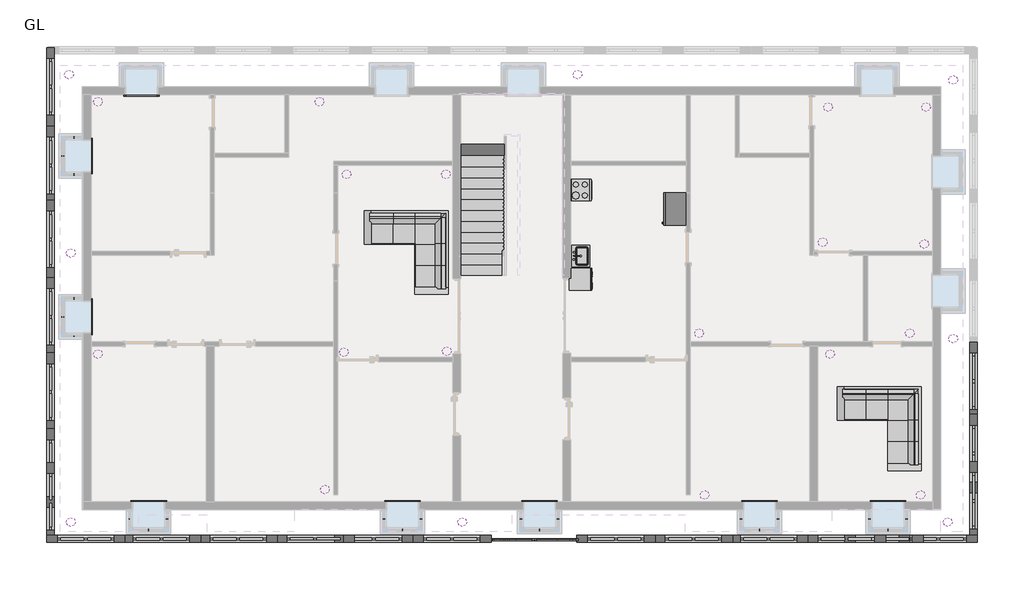
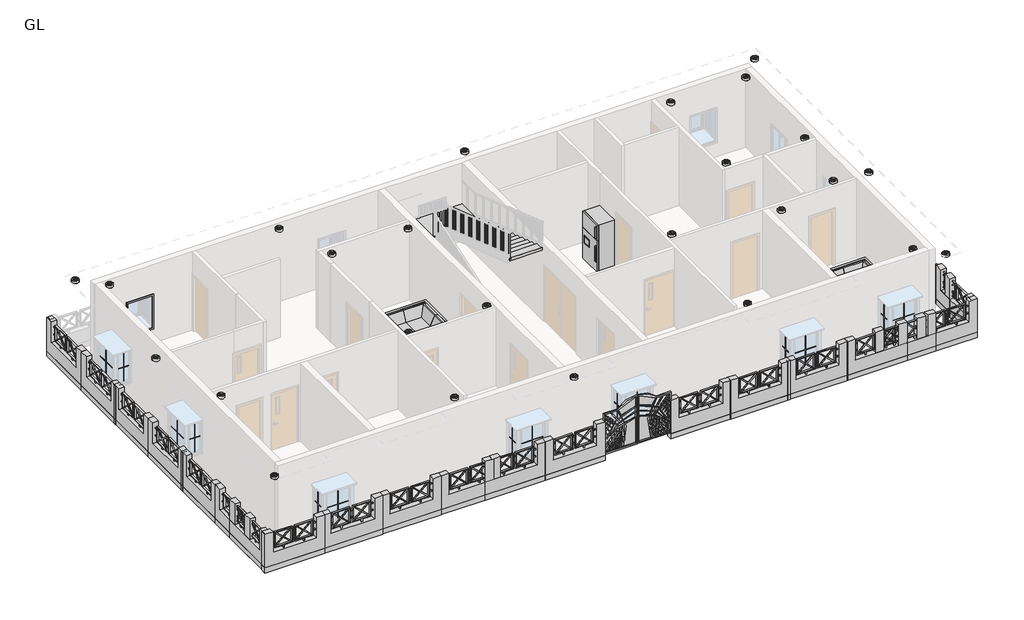
# One storey, part 4 of 5: 54 proxies, 25 light fixtures, 3 furniture elements, 1 flow terminal, 1 stair flight.
"""IFC4 building model written with IfcOpenShell, lengths in millimetres."""

from ifc_helpers import new_model, si_unit, origin, place, context, project, spatial, transform, mapped, element, save
from components import generic_models_6bc30956, dishwasher_m_610_x_610_x_860mm_47db8dec, muntin_pattern_2x2_muntin_pattern_2x2_95b57395, muntin_pattern_2x2_muntin_pattern_2x2_f03ab90d, range_m_610_x_610mm_88bdc8d1, trim_window_interior_flat_picture_frame_e50cf7ae, boundary_wall_16328_150_79515850, m_sink_kitchen_single_760_x_535mm_2_83ebd6f4, furniture_65fa61b5, corner_sofa_2406_corner_sofa_2406_47bd3d46, ceiling_light_flat_round_60w_120v_7c4c2a52, stair_flight_1eae5bb9

model = new_model("IFC4")

# Units and contexts
model_context = context("Model", 3, world=origin())
ifc_project = project(units=[si_unit("LENGTHUNIT", "METRE", prefix="MILLI")], contexts=[model_context])

# Site, building, storey
site = spatial("IfcSite", under=ifc_project)
building = spatial("IfcBuilding", under=site)
storey = spatial("IfcBuildingStorey", under=building, Name="GL", Elevation=0.0)

# Proxies
placement = place(None, origin())
generic_models_shape = generic_models_6bc30956(model_context)
element("IfcBuildingElementProxy", 1, Name="Generic Models", at=placement, inside=storey, context=model_context, shape_type="MappedRepresentation", body=[
    mapped(generic_models_shape, transform((208.0932011, -4826.8932661, 0.0), x_axis=(1.0, 0.0, 0.0), y_axis=(0.0, 1.0, 0.0), z_axis=(0.0, 0.0, 1.0))),
])
dishwasher_m_610_x_610_x_860mm_shape = dishwasher_m_610_x_610_x_860mm_47db8dec(model_context)
element("IfcBuildingElementProxy", 2, Name="Dishwasher (M) : 610 x 610 x 860mm", ObjectType="Dishwasher (M) : 610 x 610 x 860mm", at=placement, inside=storey, context=model_context, shape_type="MappedRepresentation", body=[
    mapped(dishwasher_m_610_x_610_x_860mm_shape, transform((1770.3427659, 2072.6893122, -50.8), x_axis=(0.0, 1.0, 0.0), y_axis=(-1.0, 0.0, 0.0), z_axis=(0.0, 0.0, 1.0))),
])
muntin_pattern_2x2_muntin_pattern_2x2_shape = muntin_pattern_2x2_muntin_pattern_2x2_95b57395(model_context)
element("IfcBuildingElementProxy", 3, Name="Muntin Pattern_2x2 : Muntin Pattern_2x2", ObjectType="Muntin Pattern_2x2 : Muntin Pattern_2x2", at=placement, inside=storey, context=model_context, shape_type="MappedRepresentation", body=[
    mapped(muntin_pattern_2x2_muntin_pattern_2x2_shape, transform((-10611.7987958, -4582.4182193, 730.25), x_axis=(-1.0, 0.0, 0.0), y_axis=(0.0, -1.0, 0.0), z_axis=(0.0, 0.0, 1.0))),
])
element("IfcBuildingElementProxy", 4, Name="Muntin Pattern_2x2 : Muntin Pattern_2x2", ObjectType="Muntin Pattern_2x2 : Muntin Pattern_2x2", at=placement, inside=storey, context=model_context, shape_type="MappedRepresentation", body=[
    mapped(muntin_pattern_2x2_muntin_pattern_2x2_shape, transform((-3487.0987998, -4582.4182193, 730.25), x_axis=(-1.0, 0.0, 0.0), y_axis=(0.0, -1.0, 0.0), z_axis=(0.0, 0.0, 1.0))),
])
element("IfcBuildingElementProxy", 5, Name="Muntin Pattern_2x2 : Muntin Pattern_2x2", ObjectType="Muntin Pattern_2x2 : Muntin Pattern_2x2", at=placement, inside=storey, context=model_context, shape_type="MappedRepresentation", body=[
    mapped(muntin_pattern_2x2_muntin_pattern_2x2_shape, transform((360.4932011, -4582.4182193, 730.25), x_axis=(-1.0, 0.0, 0.0), y_axis=(0.0, -1.0, 0.0), z_axis=(0.0, 0.0, 1.0))),
])
element("IfcBuildingElementProxy", 6, Name="Muntin Pattern_2x2 : Muntin Pattern_2x2", ObjectType="Muntin Pattern_2x2 : Muntin Pattern_2x2", at=placement, inside=storey, context=model_context, shape_type="MappedRepresentation", body=[
    mapped(muntin_pattern_2x2_muntin_pattern_2x2_shape, transform((6533.2012079, -4582.4182193, 730.25), x_axis=(-1.0, 0.0, 0.0), y_axis=(0.0, -1.0, 0.0), z_axis=(0.0, 0.0, 1.0))),
])
element("IfcBuildingElementProxy", 7, Name="Muntin Pattern_2x2 : Muntin Pattern_2x2", ObjectType="Muntin Pattern_2x2 : Muntin Pattern_2x2", at=placement, inside=storey, context=model_context, shape_type="MappedRepresentation", body=[
    mapped(muntin_pattern_2x2_muntin_pattern_2x2_shape, transform((10140.0012075, -4582.4182193, 730.25), x_axis=(-1.0, 0.0, 0.0), y_axis=(0.0, -1.0, 0.0), z_axis=(0.0, 0.0, 1.0))),
])
element("IfcBuildingElementProxy", 8, Name="Muntin Pattern_2x2 : Muntin Pattern_2x2", ObjectType="Muntin Pattern_2x2 : Muntin Pattern_2x2", at=placement, inside=storey, context=model_context, shape_type="MappedRepresentation", body=[
    mapped(muntin_pattern_2x2_muntin_pattern_2x2_shape, transform((-13021.6237925, 1402.4567334, 730.25), x_axis=(0.0, 1.0, 0.0), y_axis=(-1.0, 0.0, 0.0), z_axis=(0.0, 0.0, 1.0))),
])
element("IfcBuildingElementProxy", 9, Name="Muntin Pattern_2x2 : Muntin Pattern_2x2", ObjectType="Muntin Pattern_2x2 : Muntin Pattern_2x2", at=placement, inside=storey, context=model_context, shape_type="MappedRepresentation", body=[
    mapped(muntin_pattern_2x2_muntin_pattern_2x2_shape, transform((-13021.6237925, 5917.3067329, 730.25), x_axis=(0.0, 1.0, 0.0), y_axis=(-1.0, 0.0, 0.0), z_axis=(0.0, 0.0, 1.0))),
])
muntin_pattern_2x2_muntin_pattern_2x2_2_shape = muntin_pattern_2x2_muntin_pattern_2x2_f03ab90d(model_context)
element("IfcBuildingElementProxy", 10, Name="Muntin Pattern_2x2 : Muntin Pattern_2x2", ObjectType="Muntin Pattern_2x2 : Muntin Pattern_2x2", at=placement, inside=storey, context=model_context, shape_type="MappedRepresentation", body=[
    mapped(muntin_pattern_2x2_muntin_pattern_2x2_2_shape, transform((-10094.2737958, -4268.0932193, 730.25), x_axis=(0.0, 1.0, 0.0), y_axis=(-1.0, 0.0, 0.0), z_axis=(0.0, 0.0, 1.0))),
])
element("IfcBuildingElementProxy", 11, Name="Muntin Pattern_2x2 : Muntin Pattern_2x2", ObjectType="Muntin Pattern_2x2 : Muntin Pattern_2x2", at=placement, inside=storey, context=model_context, shape_type="MappedRepresentation", body=[
    mapped(muntin_pattern_2x2_muntin_pattern_2x2_2_shape, transform((-11129.3237958, -4268.0932193, 730.25), x_axis=(0.0, -1.0, 0.0), y_axis=(1.0, 0.0, 0.0), z_axis=(0.0, 0.0, 1.0))),
])
element("IfcBuildingElementProxy", 12, Name="Muntin Pattern_2x2 : Muntin Pattern_2x2", ObjectType="Muntin Pattern_2x2 : Muntin Pattern_2x2", at=placement, inside=storey, context=model_context, shape_type="MappedRepresentation", body=[
    mapped(muntin_pattern_2x2_muntin_pattern_2x2_2_shape, transform((-2969.5737998, -4268.0932193, 730.25), x_axis=(0.0, 1.0, 0.0), y_axis=(-1.0, 0.0, 0.0), z_axis=(0.0, 0.0, 1.0))),
])
element("IfcBuildingElementProxy", 13, Name="Muntin Pattern_2x2 : Muntin Pattern_2x2", ObjectType="Muntin Pattern_2x2 : Muntin Pattern_2x2", at=placement, inside=storey, context=model_context, shape_type="MappedRepresentation", body=[
    mapped(muntin_pattern_2x2_muntin_pattern_2x2_2_shape, transform((-4004.6237998, -4268.0932193, 730.25), x_axis=(0.0, -1.0, 0.0), y_axis=(1.0, 0.0, 0.0), z_axis=(0.0, 0.0, 1.0))),
])
element("IfcBuildingElementProxy", 14, Name="Muntin Pattern_2x2 : Muntin Pattern_2x2", ObjectType="Muntin Pattern_2x2 : Muntin Pattern_2x2", at=placement, inside=storey, context=model_context, shape_type="MappedRepresentation", body=[
    mapped(muntin_pattern_2x2_muntin_pattern_2x2_2_shape, transform((878.0182011, -4268.0932193, 730.25), x_axis=(0.0, 1.0, 0.0), y_axis=(-1.0, 0.0, 0.0), z_axis=(0.0, 0.0, 1.0))),
])
element("IfcBuildingElementProxy", 15, Name="Muntin Pattern_2x2 : Muntin Pattern_2x2", ObjectType="Muntin Pattern_2x2 : Muntin Pattern_2x2", at=placement, inside=storey, context=model_context, shape_type="MappedRepresentation", body=[
    mapped(muntin_pattern_2x2_muntin_pattern_2x2_2_shape, transform((-157.0317989, -4268.0932193, 730.25), x_axis=(0.0, -1.0, 0.0), y_axis=(1.0, 0.0, 0.0), z_axis=(0.0, 0.0, 1.0))),
])
element("IfcBuildingElementProxy", 16, Name="Muntin Pattern_2x2 : Muntin Pattern_2x2", ObjectType="Muntin Pattern_2x2 : Muntin Pattern_2x2", at=placement, inside=storey, context=model_context, shape_type="MappedRepresentation", body=[
    mapped(muntin_pattern_2x2_muntin_pattern_2x2_2_shape, transform((7050.7262079, -4268.0932193, 730.25), x_axis=(0.0, 1.0, 0.0), y_axis=(-1.0, 0.0, 0.0), z_axis=(0.0, 0.0, 1.0))),
])
element("IfcBuildingElementProxy", 17, Name="Muntin Pattern_2x2 : Muntin Pattern_2x2", ObjectType="Muntin Pattern_2x2 : Muntin Pattern_2x2", at=placement, inside=storey, context=model_context, shape_type="MappedRepresentation", body=[
    mapped(muntin_pattern_2x2_muntin_pattern_2x2_2_shape, transform((6015.6762079, -4268.0932193, 730.25), x_axis=(0.0, -1.0, 0.0), y_axis=(1.0, 0.0, 0.0), z_axis=(0.0, 0.0, 1.0))),
])
element("IfcBuildingElementProxy", 18, Name="Muntin Pattern_2x2 : Muntin Pattern_2x2", ObjectType="Muntin Pattern_2x2 : Muntin Pattern_2x2", at=placement, inside=storey, context=model_context, shape_type="MappedRepresentation", body=[
    mapped(muntin_pattern_2x2_muntin_pattern_2x2_2_shape, transform((10657.5262075, -4268.0932193, 730.25), x_axis=(0.0, 1.0, 0.0), y_axis=(-1.0, 0.0, 0.0), z_axis=(0.0, 0.0, 1.0))),
])
element("IfcBuildingElementProxy", 19, Name="Muntin Pattern_2x2 : Muntin Pattern_2x2", ObjectType="Muntin Pattern_2x2 : Muntin Pattern_2x2", at=placement, inside=storey, context=model_context, shape_type="MappedRepresentation", body=[
    mapped(muntin_pattern_2x2_muntin_pattern_2x2_2_shape, transform((9622.4762075, -4268.0932193, 730.25), x_axis=(0.0, -1.0, 0.0), y_axis=(1.0, 0.0, 0.0), z_axis=(0.0, 0.0, 1.0))),
])
element("IfcBuildingElementProxy", 20, Name="Muntin Pattern_2x2 : Muntin Pattern_2x2", ObjectType="Muntin Pattern_2x2 : Muntin Pattern_2x2", at=placement, inside=storey, context=model_context, shape_type="MappedRepresentation", body=[
    mapped(muntin_pattern_2x2_muntin_pattern_2x2_2_shape, transform((-12707.2987925, 884.9317334, 730.25), x_axis=(1.0, 0.0, 0.0), y_axis=(0.0, 1.0, 0.0), z_axis=(0.0, 0.0, 1.0))),
])
element("IfcBuildingElementProxy", 21, Name="Muntin Pattern_2x2 : Muntin Pattern_2x2", ObjectType="Muntin Pattern_2x2 : Muntin Pattern_2x2", at=placement, inside=storey, context=model_context, shape_type="MappedRepresentation", body=[
    mapped(muntin_pattern_2x2_muntin_pattern_2x2_2_shape, transform((-12707.2987925, 1919.9817334, 730.25), x_axis=(-1.0, 0.0, 0.0), y_axis=(0.0, -1.0, 0.0), z_axis=(0.0, 0.0, 1.0))),
])
element("IfcBuildingElementProxy", 22, Name="Muntin Pattern_2x2 : Muntin Pattern_2x2", ObjectType="Muntin Pattern_2x2 : Muntin Pattern_2x2", at=placement, inside=storey, context=model_context, shape_type="MappedRepresentation", body=[
    mapped(muntin_pattern_2x2_muntin_pattern_2x2_2_shape, transform((-12707.2987925, 5399.7817329, 730.25), x_axis=(1.0, 0.0, 0.0), y_axis=(0.0, 1.0, 0.0), z_axis=(0.0, 0.0, 1.0))),
])
element("IfcBuildingElementProxy", 23, Name="Muntin Pattern_2x2 : Muntin Pattern_2x2", ObjectType="Muntin Pattern_2x2 : Muntin Pattern_2x2", at=placement, inside=storey, context=model_context, shape_type="MappedRepresentation", body=[
    mapped(muntin_pattern_2x2_muntin_pattern_2x2_2_shape, transform((-12707.2987925, 6434.8317329, 730.25), x_axis=(-1.0, 0.0, 0.0), y_axis=(0.0, -1.0, 0.0), z_axis=(0.0, 0.0, 1.0))),
])
range_m_610_x_610mm_shape = range_m_610_x_610mm_88bdc8d1(model_context)
element("IfcBuildingElementProxy", 24, Name="Range (M) : 610 x 610mm", ObjectType="Range (M) : 610 x 610mm", at=placement, inside=storey, context=model_context, shape_type="MappedRepresentation", body=[
    mapped(range_m_610_x_610mm_shape, transform((1808.6932011, 4657.8067807, -50.8), x_axis=(0.0, 1.0, 0.0), y_axis=(-1.0, 0.0, 0.0), z_axis=(0.0, 0.0, 1.0))),
])
trim_window_interior_flat_picture_frame_shape = trim_window_interior_flat_picture_frame_e50cf7ae(model_context)
element("IfcBuildingElementProxy", 25, Name="Trim-Window-Interior-Flat : Picture Frame", ObjectType="Trim-Window-Interior-Flat : Picture Frame", at=placement, inside=storey, context=model_context, shape_type="MappedRepresentation", body=[
    mapped(trim_window_interior_flat_picture_frame_shape, transform((-10814.9987925, 7631.8067329, 1879.6), x_axis=(1.0, 0.0, 0.0), y_axis=(0.0, 0.0, 1.0), z_axis=(0.0, -1.0, 0.0))),
])
element("IfcBuildingElementProxy", 26, Name="Trim-Window-Interior-Flat : Picture Frame", ObjectType="Trim-Window-Interior-Flat : Picture Frame", at=placement, inside=storey, context=model_context, shape_type="MappedRepresentation", body=[
    mapped(trim_window_interior_flat_picture_frame_shape, transform((-10611.7987958, -3785.4932193, 1879.6), x_axis=(-1.0, 0.0, 0.0), y_axis=(0.0, 0.0, 1.0), z_axis=(0.0, 1.0, 0.0))),
])
element("IfcBuildingElementProxy", 27, Name="Trim-Window-Interior-Flat : Picture Frame", ObjectType="Trim-Window-Interior-Flat : Picture Frame", at=placement, inside=storey, context=model_context, shape_type="MappedRepresentation", body=[
    mapped(trim_window_interior_flat_picture_frame_shape, transform((-3487.0987998, -3785.4932193, 1879.6), x_axis=(-1.0, 0.0, 0.0), y_axis=(0.0, 0.0, 1.0), z_axis=(0.0, 1.0, 0.0))),
])
element("IfcBuildingElementProxy", 28, Name="Trim-Window-Interior-Flat : Picture Frame", ObjectType="Trim-Window-Interior-Flat : Picture Frame", at=placement, inside=storey, context=model_context, shape_type="MappedRepresentation", body=[
    mapped(trim_window_interior_flat_picture_frame_shape, transform((360.4932011, -3785.4932193, 1879.6), x_axis=(-1.0, 0.0, 0.0), y_axis=(0.0, 0.0, 1.0), z_axis=(0.0, 1.0, 0.0))),
])
element("IfcBuildingElementProxy", 29, Name="Trim-Window-Interior-Flat : Picture Frame", ObjectType="Trim-Window-Interior-Flat : Picture Frame", at=placement, inside=storey, context=model_context, shape_type="MappedRepresentation", body=[
    mapped(trim_window_interior_flat_picture_frame_shape, transform((6533.2012079, -3785.4932193, 1879.6), x_axis=(-1.0, 0.0, 0.0), y_axis=(0.0, 0.0, 1.0), z_axis=(0.0, 1.0, 0.0))),
])
element("IfcBuildingElementProxy", 30, Name="Trim-Window-Interior-Flat : Picture Frame", ObjectType="Trim-Window-Interior-Flat : Picture Frame", at=placement, inside=storey, context=model_context, shape_type="MappedRepresentation", body=[
    mapped(trim_window_interior_flat_picture_frame_shape, transform((10140.0012075, -3785.4932193, 1879.6), x_axis=(-1.0, 0.0, 0.0), y_axis=(0.0, 0.0, 1.0), z_axis=(0.0, 1.0, 0.0))),
])
element("IfcBuildingElementProxy", 31, Name="Trim-Window-Interior-Flat : Picture Frame", ObjectType="Trim-Window-Interior-Flat : Picture Frame", at=placement, inside=storey, context=model_context, shape_type="MappedRepresentation", body=[
    mapped(trim_window_interior_flat_picture_frame_shape, transform((-12224.6987925, 1402.4567334, 1879.6), x_axis=(0.0, 1.0, 0.0), y_axis=(0.0, 0.0, 1.0), z_axis=(1.0, 0.0, 0.0))),
])
element("IfcBuildingElementProxy", 32, Name="Trim-Window-Interior-Flat : Picture Frame", ObjectType="Trim-Window-Interior-Flat : Picture Frame", at=placement, inside=storey, context=model_context, shape_type="MappedRepresentation", body=[
    mapped(trim_window_interior_flat_picture_frame_shape, transform((-12224.6987925, 5917.3067329, 1879.6), x_axis=(0.0, 1.0, 0.0), y_axis=(0.0, 0.0, 1.0), z_axis=(1.0, 0.0, 0.0))),
])
boundary_wall_16328_150_shape = boundary_wall_16328_150_79515850(model_context)
element("IfcBuildingElementProxy", 33, Name="boundary_wall__16328 : 150", ObjectType="boundary_wall__16328 : 150", at=placement, inside=storey, context=model_context, shape_type="MappedRepresentation", body=[
    mapped(boundary_wall_16328_150_shape, transform((-12377.0987925, -4826.8932661, 0.0), x_axis=(1.0, 0.0, 0.0), y_axis=(0.0, 1.0, 0.0), z_axis=(0.0, 0.0, 1.0))),
])
element("IfcBuildingElementProxy", 34, Name="boundary_wall__16328 : 150", ObjectType="boundary_wall__16328 : 150", at=placement, inside=storey, context=model_context, shape_type="MappedRepresentation", body=[
    mapped(boundary_wall_16328_150_shape, transform((-10256.1987992, -4826.8932661, 0.0), x_axis=(1.0, 0.0, 0.0), y_axis=(0.0, 1.0, 0.0), z_axis=(0.0, 0.0, 1.0))),
])
element("IfcBuildingElementProxy", 35, Name="boundary_wall__16328 : 150", ObjectType="boundary_wall__16328 : 150", at=placement, inside=storey, context=model_context, shape_type="MappedRepresentation", body=[
    mapped(boundary_wall_16328_150_shape, transform((-8103.5487995, -4826.8932661, 0.0), x_axis=(1.0, 0.0, 0.0), y_axis=(0.0, 1.0, 0.0), z_axis=(0.0, 0.0, 1.0))),
])
element("IfcBuildingElementProxy", 36, Name="boundary_wall__16328 : 150", ObjectType="boundary_wall__16328 : 150", at=placement, inside=storey, context=model_context, shape_type="MappedRepresentation", body=[
    mapped(boundary_wall_16328_150_shape, transform((-4293.5487995, -4826.8932661, 0.0), x_axis=(1.0, 0.0, 0.0), y_axis=(0.0, 1.0, 0.0), z_axis=(0.0, 0.0, 1.0))),
])
element("IfcBuildingElementProxy", 37, Name="boundary_wall__16328 : 150", ObjectType="boundary_wall__16328 : 150", at=placement, inside=storey, context=model_context, shape_type="MappedRepresentation", body=[
    mapped(boundary_wall_16328_150_shape, transform((11549.7012075, -4826.8932661, 0.0), x_axis=(1.0, 0.0, 0.0), y_axis=(0.0, 1.0, 0.0), z_axis=(0.0, 0.0, 1.0))),
])
element("IfcBuildingElementProxy", 38, Name="boundary_wall__16328 : 150", ObjectType="boundary_wall__16328 : 150", at=placement, inside=storey, context=model_context, shape_type="MappedRepresentation", body=[
    mapped(boundary_wall_16328_150_shape, transform((8971.6012075, -4826.8932661, 0.0), x_axis=(1.0, 0.0, 0.0), y_axis=(0.0, 1.0, 0.0), z_axis=(0.0, 0.0, 1.0))),
])
element("IfcBuildingElementProxy", 39, Name="boundary_wall__16328 : 150", ObjectType="boundary_wall__16328 : 150", at=placement, inside=storey, context=model_context, shape_type="MappedRepresentation", body=[
    mapped(boundary_wall_16328_150_shape, transform((6787.2012079, -4826.8932661, 0.0), x_axis=(1.0, 0.0, 0.0), y_axis=(0.0, 1.0, 0.0), z_axis=(0.0, 0.0, 1.0))),
])
element("IfcBuildingElementProxy", 40, Name="boundary_wall__16328 : 150", ObjectType="boundary_wall__16328 : 150", at=placement, inside=storey, context=model_context, shape_type="MappedRepresentation", body=[
    mapped(boundary_wall_16328_150_shape, transform((4679.0012079, -4826.8932661, 0.0), x_axis=(1.0, 0.0, 0.0), y_axis=(0.0, 1.0, 0.0), z_axis=(0.0, 0.0, 1.0))),
])
element("IfcBuildingElementProxy", 41, Name="boundary_wall__16328 : 150", ObjectType="boundary_wall__16328 : 150", at=placement, inside=storey, context=model_context, shape_type="MappedRepresentation", body=[
    mapped(boundary_wall_16328_150_shape, transform((2500.9512082, -4826.8932661, 0.0), x_axis=(1.0, 0.0, 0.0), y_axis=(0.0, 1.0, 0.0), z_axis=(0.0, 0.0, 1.0))),
])
element("IfcBuildingElementProxy", 42, Name="boundary_wall__16328 : 150", ObjectType="boundary_wall__16328 : 150", at=placement, inside=storey, context=model_context, shape_type="MappedRepresentation", body=[
    mapped(boundary_wall_16328_150_shape, transform((-2102.7987998, -4826.8932661, 0.0), x_axis=(1.0, 0.0, 0.0), y_axis=(0.0, 1.0, 0.0), z_axis=(0.0, 0.0, 1.0))),
])
element("IfcBuildingElementProxy", 43, Name="boundary_wall__16328 : 150", ObjectType="boundary_wall__16328 : 150", at=placement, inside=storey, context=model_context, shape_type="MappedRepresentation", body=[
    mapped(boundary_wall_16328_150_shape, transform((-5938.1987925, -4823.9421379, 0.0), x_axis=(1.0, 0.0, 0.0), y_axis=(0.0, 1.0, 0.0), z_axis=(0.0, 0.0, 1.0))),
])
element("IfcBuildingElementProxy", 44, Name="boundary_wall__16328 : 150", ObjectType="boundary_wall__16328 : 150", at=placement, inside=storey, context=model_context, shape_type="MappedRepresentation", body=[
    mapped(boundary_wall_16328_150_shape, transform((12540.3012043, -2432.9432666, 0.0), x_axis=(0.0, 1.0, 0.0), y_axis=(-1.0, 0.0, 0.0), z_axis=(0.0, 0.0, 1.0))),
])
element("IfcBuildingElementProxy", 45, Name="boundary_wall__16328 : 150", ObjectType="boundary_wall__16328 : 150", at=placement, inside=storey, context=model_context, shape_type="MappedRepresentation", body=[
    mapped(boundary_wall_16328_150_shape, transform((12540.3012043, -404.3421379, 0.0), x_axis=(0.0, 1.0, 0.0), y_axis=(-1.0, 0.0, 0.0), z_axis=(0.0, 0.0, 1.0))),
])
element("IfcBuildingElementProxy", 46, Name="boundary_wall__16328 : 150", ObjectType="boundary_wall__16328 : 150", at=placement, inside=storey, context=model_context, shape_type="MappedRepresentation", body=[
    mapped(boundary_wall_16328_150_shape, transform((-13367.6987957, 7860.4067329, 0.0), x_axis=(0.0, 1.0, 0.0), y_axis=(-1.0, 0.0, 0.0), z_axis=(0.0, 0.0, 1.0))),
])
element("IfcBuildingElementProxy", 47, Name="boundary_wall__16328 : 150", ObjectType="boundary_wall__16328 : 150", at=placement, inside=storey, context=model_context, shape_type="MappedRepresentation", body=[
    mapped(boundary_wall_16328_150_shape, transform((-13367.6987957, 5650.6067329, 0.0), x_axis=(0.0, 1.0, 0.0), y_axis=(-1.0, 0.0, 0.0), z_axis=(0.0, 0.0, 1.0))),
])
element("IfcBuildingElementProxy", 48, Name="boundary_wall__16328 : 150", ObjectType="boundary_wall__16328 : 150", at=placement, inside=storey, context=model_context, shape_type="MappedRepresentation", body=[
    mapped(boundary_wall_16328_150_shape, transform((-13367.6987957, 3574.1567329, 0.0), x_axis=(0.0, 1.0, 0.0), y_axis=(-1.0, 0.0, 0.0), z_axis=(0.0, 0.0, 1.0))),
])
element("IfcBuildingElementProxy", 49, Name="boundary_wall__16328 : 150", ObjectType="boundary_wall__16328 : 150", at=placement, inside=storey, context=model_context, shape_type="MappedRepresentation", body=[
    mapped(boundary_wall_16328_150_shape, transform((-13367.6987957, 1402.4567334, 0.0), x_axis=(0.0, 1.0, 0.0), y_axis=(-1.0, 0.0, 0.0), z_axis=(0.0, 0.0, 1.0))),
])
element("IfcBuildingElementProxy", 50, Name="boundary_wall__16328 : 150", ObjectType="boundary_wall__16328 : 150", at=placement, inside=storey, context=model_context, shape_type="MappedRepresentation", body=[
    mapped(boundary_wall_16328_150_shape, transform((-13367.6987957, -709.1421379, 0.0), x_axis=(0.0, 1.0, 0.0), y_axis=(-1.0, 0.0, 0.0), z_axis=(0.0, 0.0, 1.0))),
])
element("IfcBuildingElementProxy", 51, Name="boundary_wall__16328 : 150", ObjectType="boundary_wall__16328 : 150", at=placement, inside=storey, context=model_context, shape_type="MappedRepresentation", body=[
    mapped(boundary_wall_16328_150_shape, transform((-13367.6987957, -2842.7421379, 0.0), x_axis=(0.0, 1.0, 0.0), y_axis=(-1.0, 0.0, 0.0), z_axis=(0.0, 0.0, 1.0))),
])
element("IfcBuildingElementProxy", 52, Name="boundary_wall__16328 : 150", ObjectType="boundary_wall__16328 : 150", at=placement, inside=storey, context=model_context, shape_type="MappedRepresentation", body=[
    mapped(boundary_wall_16328_150_shape, transform((-13367.6987957, -3785.4932193, 0.0), x_axis=(0.0, 1.0, 0.0), y_axis=(-1.0, 0.0, 0.0), z_axis=(0.0, 0.0, 1.0))),
])
element("IfcBuildingElementProxy", 53, Name="boundary_wall__16328 : 150", ObjectType="boundary_wall__16328 : 150", at=placement, inside=storey, context=model_context, shape_type="MappedRepresentation", body=[
    mapped(boundary_wall_16328_150_shape, transform((12540.3012043, -3762.3432666, 0.0), x_axis=(0.0, 1.0, 0.0), y_axis=(-1.0, 0.0, 0.0), z_axis=(0.0, 0.0, 1.0))),
])
element("IfcBuildingElementProxy", 54, Name="boundary_wall__16328 : 150", ObjectType="boundary_wall__16328 : 150", at=placement, inside=storey, context=model_context, shape_type="MappedRepresentation", body=[
    mapped(boundary_wall_16328_150_shape, transform((10021.6012075, -4826.8932661, 0.0), x_axis=(1.0, 0.0, 0.0), y_axis=(0.0, 1.0, 0.0), z_axis=(0.0, 0.0, 1.0))),
])

# Flow terminal
m_sink_kitchen_single_760_x_535mm_2_shape = m_sink_kitchen_single_760_x_535mm_2_83ebd6f4(model_context)
element("IfcFlowTerminal", 55, ObjectType="M_Sink Kitchen-Single : 760 x 535mm 2", at=placement, inside=storey, context=model_context, shape_type="MappedRepresentation", body=[
    mapped(m_sink_kitchen_single_760_x_535mm_2_shape, transform((1518.7386022, 3128.4960212, -50.8), x_axis=(0.0, -1.0, 0.0), y_axis=(1.0, 0.0, 0.0), z_axis=(0.0, 0.0, 1.0))),
])

# Furniture
furniture_shape = furniture_65fa61b5(model_context)
element("IfcFurniture", 56, at=placement, inside=storey, context=model_context, shape_type="MappedRepresentation", body=[
    mapped(furniture_shape, transform((4507.551208, 3815.4567334, 0.0), x_axis=(0.0, -1.0, 0.0), y_axis=(1.0, 0.0, 0.0), z_axis=(0.0, 0.0, 1.0))),
])
corner_sofa_2406_corner_sofa_2406_shape = corner_sofa_2406_corner_sofa_2406_47bd3d46(model_context)
element("IfcFurniture", 57, ObjectType="Corner_Sofa_2406 : Corner_Sofa_2406", at=placement, inside=storey, context=model_context, shape_type="MappedRepresentation", body=[
    mapped(corner_sofa_2406_corner_sofa_2406_shape, transform((-3283.8987998, 4386.9567329, 0.0), x_axis=(1.0, 0.0, 0.0), y_axis=(0.0, 1.0, 0.0), z_axis=(0.0, 0.0, 1.0))),
])
element("IfcFurniture", 58, ObjectType="Corner_Sofa_2406 : Corner_Sofa_2406", at=placement, inside=storey, context=model_context, shape_type="MappedRepresentation", body=[
    mapped(corner_sofa_2406_corner_sofa_2406_shape, transform((9987.6012075, -556.7421379, 0.0), x_axis=(1.0, 0.0, 0.0), y_axis=(0.0, 1.0, 0.0), z_axis=(0.0, 0.0, 1.0))),
])

# Light fixtures
ceiling_light_flat_round_60w_120v_shape = ceiling_light_flat_round_60w_120v_7c4c2a52(model_context)
element("IfcLightFixture", 59, ObjectType="Ceiling Light - Flat Round : 60W - 120V", at=placement, inside=storey, context=model_context, shape_type="MappedRepresentation", body=[
    mapped(ceiling_light_flat_round_60w_120v_shape, transform((-12846.9987925, 8203.3067329, 609.6), x_axis=(1.0, 0.0, 0.0), y_axis=(0.0, 1.0, 0.0), z_axis=(0.0, 0.0, 1.0))),
])
element("IfcLightFixture", 60, ObjectType="Ceiling Light - Flat Round : 60W - 120V", at=placement, inside=storey, context=model_context, shape_type="MappedRepresentation", body=[
    mapped(ceiling_light_flat_round_60w_120v_shape, transform((-12796.1987925, 3193.1567332, 609.6), x_axis=(1.0, 0.0, 0.0), y_axis=(0.0, 1.0, 0.0), z_axis=(0.0, 0.0, 1.0))),
])
element("IfcLightFixture", 61, ObjectType="Ceiling Light - Flat Round : 60W - 120V", at=placement, inside=storey, context=model_context, shape_type="MappedRepresentation", body=[
    mapped(ceiling_light_flat_round_60w_120v_shape, transform((-12796.1987925, -4356.9932193, 609.6), x_axis=(1.0, 0.0, 0.0), y_axis=(0.0, 1.0, 0.0), z_axis=(0.0, 0.0, 1.0))),
])
element("IfcLightFixture", 62, ObjectType="Ceiling Light - Flat Round : 60W - 120V", at=placement, inside=storey, context=model_context, shape_type="MappedRepresentation", body=[
    mapped(ceiling_light_flat_round_60w_120v_shape, transform((-1810.6987998, -4356.9932193, 609.6), x_axis=(1.0, 0.0, 0.0), y_axis=(0.0, 1.0, 0.0), z_axis=(0.0, 0.0, 1.0))),
])
element("IfcLightFixture", 63, ObjectType="Ceiling Light - Flat Round : 60W - 120V", at=placement, inside=storey, context=model_context, shape_type="MappedRepresentation", body=[
    mapped(ceiling_light_flat_round_60w_120v_shape, transform((11816.4012075, -4356.9932193, 609.6), x_axis=(1.0, 0.0, 0.0), y_axis=(0.0, 1.0, 0.0), z_axis=(0.0, 0.0, 1.0))),
])
element("IfcLightFixture", 64, ObjectType="Ceiling Light - Flat Round : 60W - 120V", at=placement, inside=storey, context=model_context, shape_type="MappedRepresentation", body=[
    mapped(ceiling_light_flat_round_60w_120v_shape, transform((11968.8012075, 792.8567334, 609.6), x_axis=(1.0, 0.0, 0.0), y_axis=(0.0, 1.0, 0.0), z_axis=(0.0, 0.0, 1.0))),
])
element("IfcLightFixture", 65, ObjectType="Ceiling Light - Flat Round : 60W - 120V", at=placement, inside=storey, context=model_context, shape_type="MappedRepresentation", body=[
    mapped(ceiling_light_flat_round_60w_120v_shape, transform((11968.8012075, 8050.9067329, 609.6), x_axis=(1.0, 0.0, 0.0), y_axis=(0.0, 1.0, 0.0), z_axis=(0.0, 0.0, 1.0))),
])
element("IfcLightFixture", 66, ObjectType="Ceiling Light - Flat Round : 60W - 120V", at=placement, inside=storey, context=model_context, shape_type="MappedRepresentation", body=[
    mapped(ceiling_light_flat_round_60w_120v_shape, transform((1427.2932011, 8203.3067329, 609.6), x_axis=(1.0, 0.0, 0.0), y_axis=(0.0, 1.0, 0.0), z_axis=(0.0, 0.0, 1.0))),
])
element("IfcLightFixture", 67, ObjectType="Ceiling Light - Flat Round : 60W - 120V", at=placement, inside=storey, context=model_context, shape_type="MappedRepresentation", body=[
    mapped(ceiling_light_flat_round_60w_120v_shape, transform((4837.7512082, 945.2567334, 609.6), x_axis=(1.0, 0.0, 0.0), y_axis=(0.0, 1.0, 0.0), z_axis=(0.0, 0.0, 1.0))),
])
element("IfcLightFixture", 68, ObjectType="Ceiling Light - Flat Round : 60W - 120V", at=placement, inside=storey, context=model_context, shape_type="MappedRepresentation", body=[
    mapped(ceiling_light_flat_round_60w_120v_shape, transform((10749.6012075, 945.2567334, 609.6), x_axis=(1.0, 0.0, 0.0), y_axis=(0.0, 1.0, 0.0), z_axis=(0.0, 0.0, 1.0))),
])
element("IfcLightFixture", 69, ObjectType="Ceiling Light - Flat Round : 60W - 120V", at=placement, inside=storey, context=model_context, shape_type="MappedRepresentation", body=[
    mapped(ceiling_light_flat_round_60w_120v_shape, transform((4990.1512082, -3594.9932193, 609.6), x_axis=(1.0, 0.0, 0.0), y_axis=(0.0, 1.0, 0.0), z_axis=(0.0, 0.0, 1.0))),
])
element("IfcLightFixture", 70, ObjectType="Ceiling Light - Flat Round : 60W - 120V", at=placement, inside=storey, context=model_context, shape_type="MappedRepresentation", body=[
    mapped(ceiling_light_flat_round_60w_120v_shape, transform((11054.4012075, -3594.9932193, 609.6), x_axis=(1.0, 0.0, 0.0), y_axis=(0.0, 1.0, 0.0), z_axis=(0.0, 0.0, 1.0))),
])
element("IfcLightFixture", 71, ObjectType="Ceiling Light - Flat Round : 60W - 120V", at=placement, inside=storey, context=model_context, shape_type="MappedRepresentation", body=[
    mapped(ceiling_light_flat_round_60w_120v_shape, transform((-5055.5487995, 5402.9567329, 609.6), x_axis=(1.0, 0.0, 0.0), y_axis=(0.0, 1.0, 0.0), z_axis=(0.0, 0.0, 1.0))),
])
element("IfcLightFixture", 72, ObjectType="Ceiling Light - Flat Round : 60W - 120V", at=placement, inside=storey, context=model_context, shape_type="MappedRepresentation", body=[
    mapped(ceiling_light_flat_round_60w_120v_shape, transform((-2267.8987998, 5402.9567329, 609.6), x_axis=(1.0, 0.0, 0.0), y_axis=(0.0, 1.0, 0.0), z_axis=(0.0, 0.0, 1.0))),
])
element("IfcLightFixture", 73, ObjectType="Ceiling Light - Flat Round : 60W - 120V", at=placement, inside=storey, context=model_context, shape_type="MappedRepresentation", body=[
    mapped(ceiling_light_flat_round_60w_120v_shape, transform((-5131.7487995, 408.4578621, 609.6), x_axis=(1.0, 0.0, 0.0), y_axis=(0.0, 1.0, 0.0), z_axis=(0.0, 0.0, 1.0))),
])
element("IfcLightFixture", 74, ObjectType="Ceiling Light - Flat Round : 60W - 120V", at=placement, inside=storey, context=model_context, shape_type="MappedRepresentation", body=[
    mapped(ceiling_light_flat_round_60w_120v_shape, transform((-2242.4987998, 437.2567334, 609.6), x_axis=(1.0, 0.0, 0.0), y_axis=(0.0, 1.0, 0.0), z_axis=(0.0, 0.0, 1.0))),
])
element("IfcLightFixture", 75, ObjectType="Ceiling Light - Flat Round : 60W - 120V", at=placement, inside=storey, context=model_context, shape_type="MappedRepresentation", body=[
    mapped(ceiling_light_flat_round_60w_120v_shape, transform((8457.2512079, 7288.9067329, 609.6), x_axis=(1.0, 0.0, 0.0), y_axis=(0.0, 1.0, 0.0), z_axis=(0.0, 0.0, 1.0))),
])
element("IfcLightFixture", 76, ObjectType="Ceiling Light - Flat Round : 60W - 120V", at=placement, inside=storey, context=model_context, shape_type="MappedRepresentation", body=[
    mapped(ceiling_light_flat_round_60w_120v_shape, transform((11206.8012075, 7288.9067329, 609.6), x_axis=(1.0, 0.0, 0.0), y_axis=(0.0, 1.0, 0.0), z_axis=(0.0, 0.0, 1.0))),
])
element("IfcLightFixture", 77, ObjectType="Ceiling Light - Flat Round : 60W - 120V", at=placement, inside=storey, context=model_context, shape_type="MappedRepresentation", body=[
    mapped(ceiling_light_flat_round_60w_120v_shape, transform((8304.8512079, 3497.9567332, 609.6), x_axis=(1.0, 0.0, 0.0), y_axis=(0.0, 1.0, 0.0), z_axis=(0.0, 0.0, 1.0))),
])
element("IfcLightFixture", 78, ObjectType="Ceiling Light - Flat Round : 60W - 120V", at=placement, inside=storey, context=model_context, shape_type="MappedRepresentation", body=[
    mapped(ceiling_light_flat_round_60w_120v_shape, transform((11156.0012075, 3447.1567332, 609.6), x_axis=(1.0, 0.0, 0.0), y_axis=(0.0, 1.0, 0.0), z_axis=(0.0, 0.0, 1.0))),
])
element("IfcLightFixture", 79, ObjectType="Ceiling Light - Flat Round : 60W - 120V", at=placement, inside=storey, context=model_context, shape_type="MappedRepresentation", body=[
    mapped(ceiling_light_flat_round_60w_120v_shape, transform((8514.4012079, 357.6578621, 609.6), x_axis=(1.0, 0.0, 0.0), y_axis=(0.0, 1.0, 0.0), z_axis=(0.0, 0.0, 1.0))),
])
element("IfcLightFixture", 80, ObjectType="Ceiling Light - Flat Round : 60W - 120V", at=placement, inside=storey, context=model_context, shape_type="MappedRepresentation", body=[
    mapped(ceiling_light_flat_round_60w_120v_shape, transform((-12034.1987925, 357.6578621, 609.6), x_axis=(1.0, 0.0, 0.0), y_axis=(0.0, 1.0, 0.0), z_axis=(0.0, 0.0, 1.0))),
])
element("IfcLightFixture", 81, ObjectType="Ceiling Light - Flat Round : 60W - 120V", at=placement, inside=storey, context=model_context, shape_type="MappedRepresentation", body=[
    mapped(ceiling_light_flat_round_60w_120v_shape, transform((-12034.1987925, 7441.3067329, 609.6), x_axis=(1.0, 0.0, 0.0), y_axis=(0.0, 1.0, 0.0), z_axis=(0.0, 0.0, 1.0))),
])
element("IfcLightFixture", 82, ObjectType="Ceiling Light - Flat Round : 60W - 120V", at=placement, inside=storey, context=model_context, shape_type="MappedRepresentation", body=[
    mapped(ceiling_light_flat_round_60w_120v_shape, transform((-5817.5487995, 7441.3067329, 609.6), x_axis=(1.0, 0.0, 0.0), y_axis=(0.0, 1.0, 0.0), z_axis=(0.0, 0.0, 1.0))),
])
element("IfcLightFixture", 83, ObjectType="Ceiling Light - Flat Round : 60W - 120V", at=placement, inside=storey, context=model_context, shape_type="MappedRepresentation", body=[
    mapped(ceiling_light_flat_round_60w_120v_shape, transform((-5665.1487995, -3442.5932193, 609.6), x_axis=(1.0, 0.0, 0.0), y_axis=(0.0, 1.0, 0.0), z_axis=(0.0, 0.0, 1.0))),
])

# Stair flight
stair_flight_shape = stair_flight_1eae5bb9(model_context)
element("IfcStairFlight", 84, ObjectType="2\" Tread 1\" Nosing 1/4\" Riser", at=placement, inside=storey, context=model_context, shape_type="MappedRepresentation", body=[
    mapped(stair_flight_shape, transform((0.0, 0.0, 0.0), x_axis=(1.0, 0.0, 0.0), y_axis=(0.0, 1.0, 0.0), z_axis=(0.0, 0.0, 1.0))),
])

save(model, "model.ifc")

# Revit data of these elements
# Type
#   m.s. sheet = none
#   2" x2" pipe = none
#   1"x1"pipe = none
#   Default Elevation = 0
# Type "Dishwasher (M) : 610 x 610 x 860mm"
#   Label = "DW"
#   Depth = 2' - 0.01575"
#   Height = 2' - 9.85827"
#   Width = 2' - 0.01575"
#   Dishwasher Material = Metal - Paint Finish - Ivory,Glossy
#   Panel Face Material = Plastic - Black
#   Default Elevation = 0
# Type "Muntin Pattern_2x2 : Muntin Pattern_2x2"
#   Width [instance default] = 4' - 0"
#   Thickness = 0' - 0 1/2"
#   Height [instance default] = 4' - 0"
#   Distance = 0' - 0 3/4"
#   Interior Material [instance default] = none
#   Exterior Material [instance default] = none
#   Default Elevation = 0
# Type "Range (M) : 610 x 610mm"
#   Depth = 2' - 0.01575"
#   Width = 2' - 0.01575"
#   Burner Material = Metal - Chrome
#   Range Material = Metal - Painted Finish - Ivory,Matte
#   Default Elevation = 0
#   Assembly Code = ""
# Type "Trim-Window-Interior-Flat : Picture Frame"
#   Trim Thickness_Picture Frame = 0' - 1 1/4"
#   Trim Width = 0' - 2 1/4"
#   Trim Thickness_with Sill = 0' - 0 3/4"
#   Sill Thickness = 0' - 1 1/4"
#   Opening Width [instance default] = 2' - 0"
#   Opening Height [instance default] = 3' - 0"
#   Default Elevation = 4' - 0"
#   Sill = no
#   Picture Frame = yes
#   Trim Material [instance default] = none
# Type "boundary_wall__16328 : 150"
#   Wight Hand 2 = 0' - 11.81102"
#   Wight Hand 1 = 0' - 11.81102"
#   Void Wight = 5' - 2.99213"
#   Top.High = 2' - 7.49606"
#   F.base = 0' - 3.93701"
#   F.Wight 2 = 2' - 1.59055"
#   F.Wight 1 = 2' - 1.59055"
#   F.R = 0' - 3.93701"
#   F.L = 0' - 3.93701"
#   F.High = 1' - 11.62205"
#   Bace.High = 1' - 7.68504"
#   Default Elevation = 0
# Type "M_Sink Kitchen-Single : 760 x 535mm 2"
#   Counter Height = 3' - 0.22047"
#   Depth = 1' - 7.68504"
#   Width = 1' - 11.62205"
#   Fixture Material = Metal - Steel, Polished
#   Sink Material = Metal - Steel, Polished
#   Default Elevation = 0
#   Assembly Code = ""
# Type
#   Default Elevation = 0
# Type "Corner_Sofa_2406 : Corner_Sofa_2406"
#   Fabric = none
#   Default Elevation = 0
# Type "Ceiling Light - Flat Round : 60W - 120V"
#   Lamp = "A-19"
#   Assembly Code = "D5020220"
#   Wattage = 60 W
#   built-in parameter 1150110 = 1 (stored number, unit not read)
#   built-in parameter 1114217 = 1 (stored number, unit not read)
#   built-in parameter 1150109 = 1 (stored number, unit not read)
#   built-in parameter 1150113 = 1 (stored number, unit not read)
#   built-in parameter 1150115 = 1 (stored number, unit not read)
#   built-in parameter 1150105 = 272.155 (stored number, unit not read)
#   Light Source Symbol Size = 2' - 0"
#   built-in parameter 1150112 = 1 (stored number, unit not read)
#   built-in parameter 1150114 = 1 (stored number, unit not read)
#   built-in parameter 1150107 = 2800 (stored number, unit not read)
#   built-in parameter 1150106 = 2.72155 (stored number, unit not read)
#   Emit from Circle Diameter = 0' - 10"
#   built-in parameter 1150104 = 1.32387 (stored number, unit not read)
#   Ballast Voltage = 120 V
#   built-in parameter 1114218 = 1 (stored number, unit not read)
#   built-in parameter 1150133 = 10 (stored number, unit not read)
#   Lumens = 855 lm
#   Apparent Load = 60 VA
#   built-in parameter 1150134 = 4
#   built-in parameter 1150137 = 1
#   Color Filter = 16777215
#   built-in parameter 1140040 [instance default] = 1
#   Ballast Number of Poles = 1
#   Light Box Material = Steel, Paint Finish, Dark Gray, Matte
#   Diffuser Material = Glass, White, High Luminance
#   Wattage Comments = ""
#   Emit Shape Visible in Rendering = no
#   Dimming Lamp Color Temperature Shift = (empty or 0)
#   Default Elevation = 0
# Element 1 (IfcBuildingElementProxy)
#   Phase Created = New Construction
# Element 2 (IfcBuildingElementProxy, "Dishwasher (M) : 610 x 610 x 860mm")
#   Phase Created = New Construction
#   Materials on its faces: "Metal - Paint Finish - Ivory,Glossy", "Plastic - Black"
# Elements 3, 4, 5, 6, 7, 8, 9 (IfcBuildingElementProxy, "Muntin Pattern_2x2 : Muntin Pattern_2x2")
#   Width = 2' - 6 1/2"
#   Height = 3' - 6 1/2"
#   Interior Material = Wood - Stained
#   Exterior Material = Clad - White
#   Phase Created = New Construction
#   Materials on its faces: "Clad - White", "Wood - Stained"
# Elements 10, 11, 12, 13, 14, 15, 16, 17, 18, 19, 20, 21, 22, 23 (IfcBuildingElementProxy, "Muntin Pattern_2x2 : Muntin Pattern_2x2")
#   Width = 1' - 2 1/2"
#   Height = 3' - 6 1/2"
#   Interior Material = Wood - Stained
#   Exterior Material = Clad - White
#   Phase Created = New Construction
#   Materials on its faces: "Clad - White", "Wood - Stained"
# Element 24 (IfcBuildingElementProxy, "Range (M) : 610 x 610mm")
#   Phase Created = New Construction
#   Materials on its faces: "Metal - Painted Finish - Ivory,Matte", "Metal - Chrome", "Glass"
# Elements 25, 26, 27, 28, 29, 30, 31, 32 (IfcBuildingElementProxy, "Trim-Window-Interior-Flat : Picture Frame")
#   Opening Width = 3' - 0"
#   Opening Height = 4' - 2"
#   Trim Material = Wood - Stained
#   Phase Created = New Construction
#   Materials on its faces: "Wood - Stained"
# Elements 33, 34, 35, 36, 37, 38, 39, 40, 41, 42, 43, 44, 45, 46, 47, 48, 49, 50, 51, 52, 53, 54 (IfcBuildingElementProxy, "boundary_wall__16328 : 150")
#   Phase Created = New Construction
#   Materials on its faces: "Metal"
# Element 55 (IfcFlowTerminal, "M_Sink Kitchen-Single : 760 x 535mm 2")
#   Mark = "1"
#   Phase Created = New Construction
#   Materials on its faces: "Metal - Steel, Polished"
# Element 56 (IfcFurniture)
#   Phase Created = New Construction
#   Materials on its faces: "Default", "Default 3", "Default 2"
# Elements 57, 58 (IfcFurniture, "Corner_Sofa_2406 : Corner_Sofa_2406")
#   Phase Created = New Construction
#   Materials on its faces: "Default Wall"
# Element 59 (IfcLightFixture, "Ceiling Light - Flat Round : 60W - 120V")
#   Mark = "3"
#   built-in parameter 1140040 = 1
#   Phase Created = New Construction
#   Materials on its faces: "Glass, White, High Luminance", "Steel, Paint Finish, Dark Gray, Matte"
# Element 60 (IfcLightFixture, "Ceiling Light - Flat Round : 60W - 120V")
#   Mark = "4"
#   built-in parameter 1140040 = 1
#   Phase Created = New Construction
#   Materials on its faces: "Glass, White, High Luminance", "Steel, Paint Finish, Dark Gray, Matte"
# Element 61 (IfcLightFixture, "Ceiling Light - Flat Round : 60W - 120V")
#   Mark = "5"
#   built-in parameter 1140040 = 1
#   Phase Created = New Construction
#   Materials on its faces: "Glass, White, High Luminance", "Steel, Paint Finish, Dark Gray, Matte"
# Element 62 (IfcLightFixture, "Ceiling Light - Flat Round : 60W - 120V")
#   Mark = "6"
#   built-in parameter 1140040 = 1
#   Phase Created = New Construction
#   Materials on its faces: "Glass, White, High Luminance", "Steel, Paint Finish, Dark Gray, Matte"
# Element 63 (IfcLightFixture, "Ceiling Light - Flat Round : 60W - 120V")
#   Mark = "7"
#   built-in parameter 1140040 = 1
#   Phase Created = New Construction
#   Materials on its faces: "Glass, White, High Luminance", "Steel, Paint Finish, Dark Gray, Matte"
# Element 64 (IfcLightFixture, "Ceiling Light - Flat Round : 60W - 120V")
#   Mark = "8"
#   built-in parameter 1140040 = 1
#   Phase Created = New Construction
#   Materials on its faces: "Glass, White, High Luminance", "Steel, Paint Finish, Dark Gray, Matte"
# Element 65 (IfcLightFixture, "Ceiling Light - Flat Round : 60W - 120V")
#   Mark = "9"
#   built-in parameter 1140040 = 1
#   Phase Created = New Construction
#   Materials on its faces: "Glass, White, High Luminance", "Steel, Paint Finish, Dark Gray, Matte"
# Element 66 (IfcLightFixture, "Ceiling Light - Flat Round : 60W - 120V")
#   Mark = "10"
#   built-in parameter 1140040 = 1
#   Phase Created = New Construction
#   Materials on its faces: "Glass, White, High Luminance", "Steel, Paint Finish, Dark Gray, Matte"
# Element 67 (IfcLightFixture, "Ceiling Light - Flat Round : 60W - 120V")
#   Mark = "11"
#   built-in parameter 1140040 = 1
#   Phase Created = New Construction
#   Materials on its faces: "Glass, White, High Luminance", "Steel, Paint Finish, Dark Gray, Matte"
# Element 68 (IfcLightFixture, "Ceiling Light - Flat Round : 60W - 120V")
#   Mark = "12"
#   built-in parameter 1140040 = 1
#   Phase Created = New Construction
#   Materials on its faces: "Glass, White, High Luminance", "Steel, Paint Finish, Dark Gray, Matte"
# Element 69 (IfcLightFixture, "Ceiling Light - Flat Round : 60W - 120V")
#   Mark = "13"
#   built-in parameter 1140040 = 1
#   Phase Created = New Construction
#   Materials on its faces: "Glass, White, High Luminance", "Steel, Paint Finish, Dark Gray, Matte"
# Element 70 (IfcLightFixture, "Ceiling Light - Flat Round : 60W - 120V")
#   Mark = "14"
#   built-in parameter 1140040 = 1
#   Phase Created = New Construction
#   Materials on its faces: "Glass, White, High Luminance", "Steel, Paint Finish, Dark Gray, Matte"
# Element 71 (IfcLightFixture, "Ceiling Light - Flat Round : 60W - 120V")
#   Mark = "15"
#   built-in parameter 1140040 = 1
#   Phase Created = New Construction
#   Materials on its faces: "Glass, White, High Luminance", "Steel, Paint Finish, Dark Gray, Matte"
# Element 72 (IfcLightFixture, "Ceiling Light - Flat Round : 60W - 120V")
#   Mark = "16"
#   built-in parameter 1140040 = 1
#   Phase Created = New Construction
#   Materials on its faces: "Glass, White, High Luminance", "Steel, Paint Finish, Dark Gray, Matte"
# Element 73 (IfcLightFixture, "Ceiling Light - Flat Round : 60W - 120V")
#   Mark = "17"
#   built-in parameter 1140040 = 1
#   Phase Created = New Construction
#   Materials on its faces: "Glass, White, High Luminance", "Steel, Paint Finish, Dark Gray, Matte"
# Element 74 (IfcLightFixture, "Ceiling Light - Flat Round : 60W - 120V")
#   Mark = "18"
#   built-in parameter 1140040 = 1
#   Phase Created = New Construction
#   Materials on its faces: "Glass, White, High Luminance", "Steel, Paint Finish, Dark Gray, Matte"
# Element 75 (IfcLightFixture, "Ceiling Light - Flat Round : 60W - 120V")
#   Mark = "19"
#   built-in parameter 1140040 = 1
#   Phase Created = New Construction
#   Materials on its faces: "Glass, White, High Luminance", "Steel, Paint Finish, Dark Gray, Matte"
# Element 76 (IfcLightFixture, "Ceiling Light - Flat Round : 60W - 120V")
#   Mark = "20"
#   built-in parameter 1140040 = 1
#   Phase Created = New Construction
#   Materials on its faces: "Glass, White, High Luminance", "Steel, Paint Finish, Dark Gray, Matte"
# Element 77 (IfcLightFixture, "Ceiling Light - Flat Round : 60W - 120V")
#   Mark = "21"
#   built-in parameter 1140040 = 1
#   Phase Created = New Construction
#   Materials on its faces: "Glass, White, High Luminance", "Steel, Paint Finish, Dark Gray, Matte"
# Element 78 (IfcLightFixture, "Ceiling Light - Flat Round : 60W - 120V")
#   Mark = "22"
#   built-in parameter 1140040 = 1
#   Phase Created = New Construction
#   Materials on its faces: "Glass, White, High Luminance", "Steel, Paint Finish, Dark Gray, Matte"
# Element 79 (IfcLightFixture, "Ceiling Light - Flat Round : 60W - 120V")
#   Mark = "23"
#   built-in parameter 1140040 = 1
#   Phase Created = New Construction
#   Materials on its faces: "Glass, White, High Luminance", "Steel, Paint Finish, Dark Gray, Matte"
# Element 80 (IfcLightFixture, "Ceiling Light - Flat Round : 60W - 120V")
#   Mark = "24"
#   built-in parameter 1140040 = 1
#   Phase Created = New Construction
#   Materials on its faces: "Glass, White, High Luminance", "Steel, Paint Finish, Dark Gray, Matte"
# Element 81 (IfcLightFixture, "Ceiling Light - Flat Round : 60W - 120V")
#   Mark = "25"
#   built-in parameter 1140040 = 1
#   Phase Created = New Construction
#   Materials on its faces: "Glass, White, High Luminance", "Steel, Paint Finish, Dark Gray, Matte"
# Element 82 (IfcLightFixture, "Ceiling Light - Flat Round : 60W - 120V")
#   Mark = "26"
#   built-in parameter 1140040 = 1
#   Phase Created = New Construction
#   Materials on its faces: "Glass, White, High Luminance", "Steel, Paint Finish, Dark Gray, Matte"
# Element 83 (IfcLightFixture, "Ceiling Light - Flat Round : 60W - 120V")
#   Mark = "27"
#   built-in parameter 1140040 = 1
#   Phase Created = New Construction
#   Materials on its faces: "Glass, White, High Luminance", "Steel, Paint Finish, Dark Gray, Matte"
# Element 84 (IfcStairFlight, "2\" Tread 1\" Nosing 1/4\" Riser")
#   Phase Created = New Construction
# Materials
#   "Metal - Paint Finish - Ivory,Glossy": colour RGB 247 247 239, transparency 0
#   "Plastic - Black": colour RGB 0 0 0, transparency 0.7
#   "Metal - Chrome": colour RGB 17 17 17, transparency 0
#   "Metal - Painted Finish - Ivory,Matte": colour RGB 247 247 239, transparency 0
#   "Metal - Steel, Polished": class "Metal", colour RGB 192 192 192, transparency 0
#   "Steel, Paint Finish, Dark Gray, Matte": class "Metal", colour RGB 98 98 98, transparency 0, Description = "Steel, paint finish, dark gray, matte", Cost = 0
#   "Glass, White, High Luminance": class "Glass", colour RGB 249 250 249, transparency 0.8, Description = "physical material", Cost = 0
#   "Clad - White": class "Wood", colour RGB 242 242 238, transparency 0, Cost = 0
#   "Wood - Stained": class "Wood", colour RGB 224 178 126, transparency 0, Cost = 0
#   "Glass": class "Glass", colour RGB 0 128 192, transparency 0.75, Description = "Soda Lime Glass", Cost = 0
#   "Metal": class "Generic", colour RGB 65 64 62, transparency 0, Cost = 0
#   "Default": colour RGB 127 127 127, transparency 0, Cost = 0
#   "Default 3": class "Glass", colour RGB 127 127 127, transparency 0
#   "Default 2": class "Plastic", colour RGB 127 127 127, transparency 0
#   "Default Wall": colour RGB 128 128 128, transparency 0, Cost = 0
